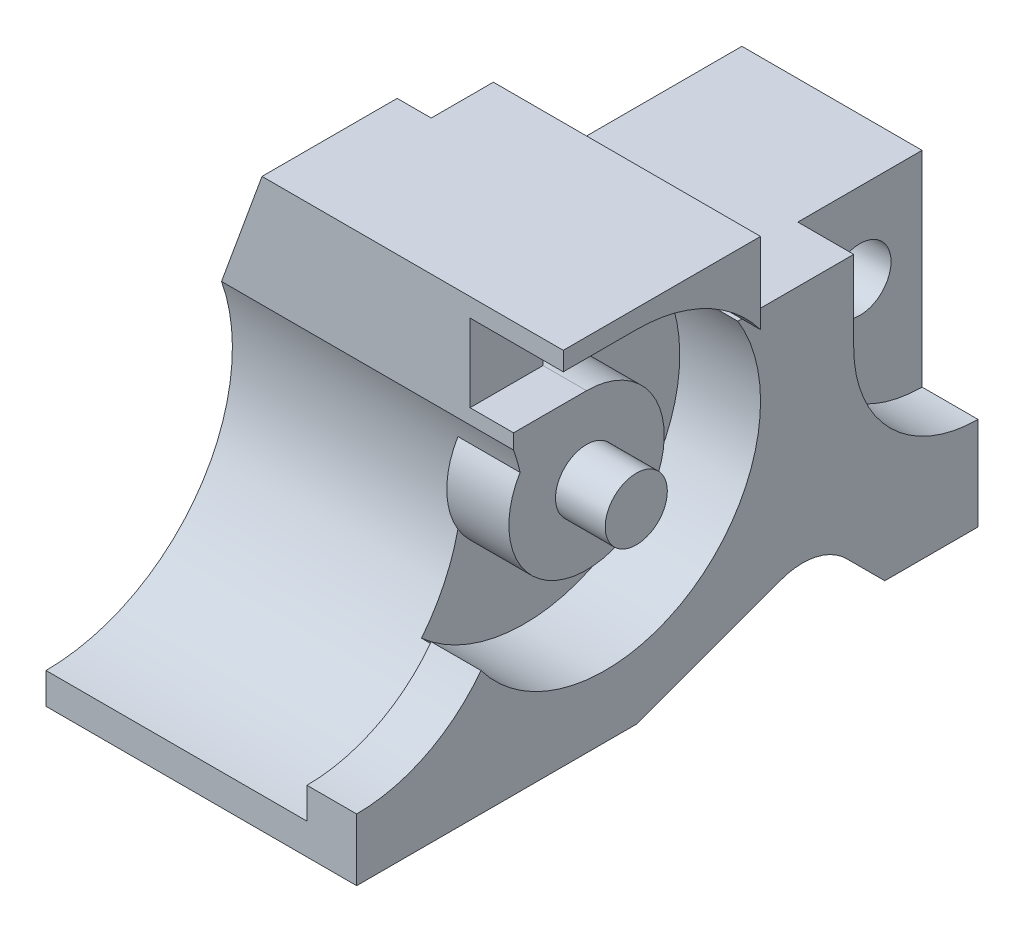
ISO-10303-21;
HEADER;
FILE_DESCRIPTION(('STEP AP214'),'2;1');
FILE_NAME('part.step','',(''),(''),'','','');
FILE_SCHEMA(('AUTOMOTIVE_DESIGN { 1 0 10303 214 1 1 1 1 }'));
ENDSEC;
DATA;
#1=APPLICATION_CONTEXT('core data for automotive mechanical design processes');
#2=APPLICATION_PROTOCOL_DEFINITION('international standard','automotive_design',2000,#1);
#3=PRODUCT_CONTEXT('',#1,'mechanical');
#4=PRODUCT('Part','Part','',(#3));
#5=PRODUCT_RELATED_PRODUCT_CATEGORY('part','',(#4));
#6=PRODUCT_DEFINITION_FORMATION('','',#4);
#7=PRODUCT_DEFINITION_CONTEXT('part definition',#1,'design');
#8=PRODUCT_DEFINITION('design','',#6,#7);
#9=PRODUCT_DEFINITION_SHAPE('','',#8);
#10=(LENGTH_UNIT() NAMED_UNIT(*) SI_UNIT(.MILLI.,.METRE.));
#11=(NAMED_UNIT(*) PLANE_ANGLE_UNIT() SI_UNIT($,.RADIAN.));
#12=(NAMED_UNIT(*) SI_UNIT($,.STERADIAN.) SOLID_ANGLE_UNIT());
#13=UNCERTAINTY_MEASURE_WITH_UNIT(LENGTH_MEASURE(1.E-05),#10,'distance_accuracy_value','');
#14=(GEOMETRIC_REPRESENTATION_CONTEXT(3) GLOBAL_UNCERTAINTY_ASSIGNED_CONTEXT((#13)) GLOBAL_UNIT_ASSIGNED_CONTEXT((#10,
#11,#12)) REPRESENTATION_CONTEXT('',''));
#15=CARTESIAN_POINT('',(0.,0.,0.));
#16=DIRECTION('',(0.,0.,1.));
#17=DIRECTION('',(1.,0.,0.));
#18=AXIS2_PLACEMENT_3D('',#15,#16,#17);
#19=CARTESIAN_POINT('',(12.,35.,-40.));
#20=DIRECTION('',(0.,0.,1.));
#21=DIRECTION('',(1.,0.,0.));
#22=AXIS2_PLACEMENT_3D('',#19,#20,#21);
#23=PLANE('',#22);
#24=DIRECTION('',(0.,-1.,0.));
#25=VECTOR('',#24,1.);
#26=CARTESIAN_POINT('',(15.,47.5,-40.));
#27=LINE('',#26,#25);
#28=CARTESIAN_POINT('',(15.,60.,-40.));
#29=VERTEX_POINT('',#28);
#30=CARTESIAN_POINT('',(15.,47.5,-40.));
#31=VERTEX_POINT('',#30);
#32=EDGE_CURVE('E259',#29,#31,#27,.T.);
#33=ORIENTED_EDGE('',*,*,#32,.T.);
#34=DIRECTION('',(-1.,0.,0.));
#35=VECTOR('',#34,1.);
#36=CARTESIAN_POINT('',(22.,47.5,-40.));
#37=LINE('',#36,#35);
#38=CARTESIAN_POINT('',(12.,47.5,-40.));
#39=VERTEX_POINT('',#38);
#40=EDGE_CURVE('E53',#39,#31,#37,.F.);
#41=ORIENTED_EDGE('',*,*,#40,.F.);
#42=DIRECTION('',(0.,-1.,0.));
#43=VECTOR('',#42,1.);
#44=CARTESIAN_POINT('',(12.,35.,-40.));
#45=LINE('',#44,#43);
#46=CARTESIAN_POINT('',(12.,60.,-40.));
#47=VERTEX_POINT('',#46);
#48=EDGE_CURVE('E308',#47,#39,#45,.T.);
#49=ORIENTED_EDGE('',*,*,#48,.F.);
#50=DIRECTION('',(1.,0.,0.));
#51=VECTOR('',#50,1.);
#52=CARTESIAN_POINT('',(12.,60.,-40.));
#53=LINE('',#52,#51);
#54=EDGE_CURVE('E312',#47,#29,#53,.T.);
#55=ORIENTED_EDGE('',*,*,#54,.T.);
#56=EDGE_LOOP('',(#33,#41,#49,#55));
#57=FACE_BOUND('',#56,.T.);
#58=ADVANCED_FACE('F46',(#57),#23,.F.);
#59=CARTESIAN_POINT('',(-25.,35.,0.));
#60=DIRECTION('',(1.,0.,0.));
#61=DIRECTION('',(0.,0.,-1.));
#62=AXIS2_PLACEMENT_3D('',#59,#60,#61);
#63=CYLINDRICAL_SURFACE('',#62,30.);
#64=CARTESIAN_POINT('',(22.,35.,0.));
#65=DIRECTION('',(-1.,0.,0.));
#66=DIRECTION('',(0.,0.,-1.));
#67=AXIS2_PLACEMENT_3D('',#64,#65,#66);
#68=CIRCLE('',#67,30.);
#69=CARTESIAN_POINT('',(22.,45.0964102531544,-28.25));
#70=VERTEX_POINT('',#69);
#71=CARTESIAN_POINT('',(22.,41.4570206159168,-29.296875));
#72=VERTEX_POINT('',#71);
#73=EDGE_CURVE('E274',#70,#72,#68,.T.);
#74=ORIENTED_EDGE('',*,*,#73,.F.);
#75=DIRECTION('',(1.,0.,0.));
#76=VECTOR('',#75,1.);
#77=CARTESIAN_POINT('',(-25.,45.0964102531544,-28.25));
#78=LINE('',#77,#76);
#79=CARTESIAN_POINT('',(-25.,45.0964102531544,-28.25));
#80=VERTEX_POINT('',#79);
#81=EDGE_CURVE('E68',#70,#80,#78,.F.);
#82=ORIENTED_EDGE('',*,*,#81,.T.);
#83=CARTESIAN_POINT('',(-25.,35.,0.));
#84=DIRECTION('',(1.,0.,0.));
#85=DIRECTION('',(0.,0.,-1.));
#86=AXIS2_PLACEMENT_3D('',#83,#84,#85);
#87=CIRCLE('',#86,30.);
#88=CARTESIAN_POINT('',(-25.,5.,0.));
#89=VERTEX_POINT('',#88);
#90=EDGE_CURVE('E348',#89,#80,#87,.T.);
#91=ORIENTED_EDGE('',*,*,#90,.F.);
#92=DIRECTION('',(1.,0.,0.));
#93=VECTOR('',#92,1.);
#94=CARTESIAN_POINT('',(-25.,5.,0.));
#95=LINE('',#94,#93);
#96=CARTESIAN_POINT('',(17.,5.,0.));
#97=VERTEX_POINT('',#96);
#98=EDGE_CURVE('E355',#89,#97,#95,.T.);
#99=ORIENTED_EDGE('',*,*,#98,.T.);
#100=CARTESIAN_POINT('',(17.,35.,0.));
#101=DIRECTION('',(1.,0.,0.));
#102=DIRECTION('',(0.,0.,-1.));
#103=AXIS2_PLACEMENT_3D('',#100,#101,#102);
#104=CIRCLE('',#103,30.);
#105=CARTESIAN_POINT('',(17.,16.2734521667767,-23.4375));
#106=VERTEX_POINT('',#105);
#107=EDGE_CURVE('E351',#97,#106,#104,.T.);
#108=ORIENTED_EDGE('',*,*,#107,.T.);
#109=DIRECTION('',(1.,0.,0.));
#110=VECTOR('',#109,1.);
#111=CARTESIAN_POINT('',(18.5,16.2734521667767,-23.4375));
#112=LINE('',#111,#110);
#113=CARTESIAN_POINT('',(12.,16.2734521667767,-23.4375));
#114=VERTEX_POINT('',#113);
#115=EDGE_CURVE('E314',#106,#114,#112,.F.);
#116=ORIENTED_EDGE('',*,*,#115,.T.);
#117=CARTESIAN_POINT('',(12.,35.,0.));
#118=DIRECTION('',(1.,0.,0.));
#119=DIRECTION('',(0.,0.,-1.));
#120=AXIS2_PLACEMENT_3D('',#117,#118,#119);
#121=CIRCLE('',#120,30.);
#122=CARTESIAN_POINT('',(12.,28.5429793840832,-29.296875));
#123=VERTEX_POINT('',#122);
#124=EDGE_CURVE('E476',#123,#114,#121,.F.);
#125=ORIENTED_EDGE('',*,*,#124,.F.);
#126=CARTESIAN_POINT('',(12.,41.4570206159168,-29.296875));
#127=VERTEX_POINT('',#126);
#128=EDGE_CURVE('E480',#127,#123,#121,.F.);
#129=ORIENTED_EDGE('',*,*,#128,.F.);
#130=DIRECTION('',(-1.,0.,0.));
#131=VECTOR('',#130,1.);
#132=CARTESIAN_POINT('',(17.,41.4570206159168,-29.296875));
#133=LINE('',#132,#131);
#134=EDGE_CURVE('E299',#72,#127,#133,.T.);
#135=ORIENTED_EDGE('',*,*,#134,.F.);
#136=EDGE_LOOP('',(#74,#82,#91,#99,#108,#116,#125,#129,#135));
#137=FACE_BOUND('',#136,.T.);
#138=ADVANCED_FACE('F521',(#137),#63,.F.);
#139=CARTESIAN_POINT('',(25.,63.,0.));
#140=DIRECTION('',(0.,1.,0.));
#141=DIRECTION('',(0.,0.,1.));
#142=AXIS2_PLACEMENT_3D('',#139,#140,#141);
#143=PLANE('',#142);
#144=DIRECTION('',(1.,0.,0.));
#145=VECTOR('',#144,1.);
#146=CARTESIAN_POINT('',(-25.,63.,-50.));
#147=LINE('',#146,#145);
#148=CARTESIAN_POINT('',(-18.4836262456348,63.,-50.));
#149=VERTEX_POINT('',#148);
#150=CARTESIAN_POINT('',(-13.,63.,-50.));
#151=VERTEX_POINT('',#150);
#152=EDGE_CURVE('E385',#149,#151,#147,.T.);
#153=ORIENTED_EDGE('',*,*,#152,.F.);
#154=DIRECTION('',(0.,0.,1.));
#155=VECTOR('',#154,1.);
#156=CARTESIAN_POINT('',(-18.4836262456348,63.,-100.));
#157=LINE('',#156,#155);
#158=CARTESIAN_POINT('',(-18.4836262456348,63.,-28.25));
#159=VERTEX_POINT('',#158);
#160=EDGE_CURVE('E332',#149,#159,#157,.T.);
#161=ORIENTED_EDGE('',*,*,#160,.T.);
#162=DIRECTION('',(-1.,0.,0.));
#163=VECTOR('',#162,1.);
#164=CARTESIAN_POINT('',(25.,63.,-28.25));
#165=LINE('',#164,#163);
#166=CARTESIAN_POINT('',(30.,63.,-28.25));
#167=VERTEX_POINT('',#166);
#168=EDGE_CURVE('E338',#167,#159,#165,.T.);
#169=ORIENTED_EDGE('',*,*,#168,.F.);
#170=DIRECTION('',(0.,0.,1.));
#171=VECTOR('',#170,1.);
#172=CARTESIAN_POINT('',(30.,63.,-28.25));
#173=LINE('',#172,#171);
#174=CARTESIAN_POINT('',(30.,63.,-60.));
#175=VERTEX_POINT('',#174);
#176=EDGE_CURVE('E273',#175,#167,#173,.T.);
#177=ORIENTED_EDGE('',*,*,#176,.F.);
#178=DIRECTION('',(1.,0.,0.));
#179=VECTOR('',#178,1.);
#180=CARTESIAN_POINT('',(-13.,63.,-60.));
#181=LINE('',#180,#179);
#182=CARTESIAN_POINT('',(-13.,63.,-60.));
#183=VERTEX_POINT('',#182);
#184=EDGE_CURVE('E370',#183,#175,#181,.T.);
#185=ORIENTED_EDGE('',*,*,#184,.F.);
#186=DIRECTION('',(0.,0.,-1.));
#187=VECTOR('',#186,1.);
#188=CARTESIAN_POINT('',(-13.,63.,-100.));
#189=LINE('',#188,#187);
#190=EDGE_CURVE('E389',#151,#183,#189,.T.);
#191=ORIENTED_EDGE('',*,*,#190,.F.);
#192=EDGE_LOOP('',(#153,#161,#169,#177,#185,#191));
#193=FACE_BOUND('',#192,.T.);
#194=ADVANCED_FACE('F503',(#193),#143,.T.);
#195=CARTESIAN_POINT('',(-25.,0.,0.));
#196=DIRECTION('',(1.,0.,0.));
#197=DIRECTION('',(0.,0.,-1.));
#198=AXIS2_PLACEMENT_3D('',#195,#196,#197);
#199=PLANE('',#198);
#200=DIRECTION('',(0.,0.,1.));
#201=VECTOR('',#200,1.);
#202=CARTESIAN_POINT('',(-25.,45.0964102531544,-100.));
#203=LINE('',#202,#201);
#204=CARTESIAN_POINT('',(-25.,45.0964102531544,-50.));
#205=VERTEX_POINT('',#204);
#206=EDGE_CURVE('E331',#205,#80,#203,.T.);
#207=ORIENTED_EDGE('',*,*,#206,.F.);
#208=DIRECTION('',(0.,-1.,0.));
#209=VECTOR('',#208,1.);
#210=CARTESIAN_POINT('',(-25.,0.,-50.));
#211=LINE('',#210,#209);
#212=CARTESIAN_POINT('',(-25.,1.81985117133101,-50.));
#213=VERTEX_POINT('',#212);
#214=EDGE_CURVE('E462',#205,#213,#211,.T.);
#215=ORIENTED_EDGE('',*,*,#214,.T.);
#216=DIRECTION('',(0.,0.34202014332567,-0.939692620785908));
#217=VECTOR('',#216,1.);
#218=CARTESIAN_POINT('',(-25.,-14.4627212179472,-5.26400002982302));
#219=LINE('',#218,#217);
#220=CARTESIAN_POINT('',(-25.,0.,-45.));
#221=VERTEX_POINT('',#220);
#222=EDGE_CURVE('E428',#221,#213,#219,.T.);
#223=ORIENTED_EDGE('',*,*,#222,.F.);
#224=DIRECTION('',(0.,0.,-1.));
#225=VECTOR('',#224,1.);
#226=CARTESIAN_POINT('',(-25.,0.,0.));
#227=LINE('',#226,#225);
#228=CARTESIAN_POINT('',(-25.,0.,0.));
#229=VERTEX_POINT('',#228);
#230=EDGE_CURVE('E444',#229,#221,#227,.T.);
#231=ORIENTED_EDGE('',*,*,#230,.F.);
#232=DIRECTION('',(0.,1.,0.));
#233=VECTOR('',#232,1.);
#234=CARTESIAN_POINT('',(-25.,0.,0.));
#235=LINE('',#234,#233);
#236=EDGE_CURVE('E419',#229,#89,#235,.T.);
#237=ORIENTED_EDGE('',*,*,#236,.T.);
#238=ORIENTED_EDGE('',*,*,#90,.T.);
#239=EDGE_LOOP('',(#207,#215,#223,#231,#237,#238));
#240=FACE_BOUND('',#239,.T.);
#241=ADVANCED_FACE('F519',(#240),#199,.F.);
#242=CARTESIAN_POINT('',(-25.,0.,-50.));
#243=DIRECTION('',(0.,0.,1.));
#244=DIRECTION('',(1.,0.,0.));
#245=AXIS2_PLACEMENT_3D('',#242,#243,#244);
#246=PLANE('',#245);
#247=DIRECTION('',(-0.342020143325663,-0.939692620785911,0.));
#248=VECTOR('',#247,1.);
#249=CARTESIAN_POINT('',(-39.4937068760341,5.2752778870557,-50.));
#250=LINE('',#249,#248);
#251=EDGE_CURVE('E336',#149,#205,#250,.T.);
#252=ORIENTED_EDGE('',*,*,#251,.F.);
#253=ORIENTED_EDGE('',*,*,#152,.T.);
#254=DIRECTION('',(0.,1.,0.));
#255=VECTOR('',#254,1.);
#256=CARTESIAN_POINT('',(-13.,0.,-50.));
#257=LINE('',#256,#255);
#258=CARTESIAN_POINT('',(-13.,1.81985117133101,-50.));
#259=VERTEX_POINT('',#258);
#260=EDGE_CURVE('E388',#259,#151,#257,.T.);
#261=ORIENTED_EDGE('',*,*,#260,.F.);
#262=DIRECTION('',(1.,0.,0.));
#263=VECTOR('',#262,1.);
#264=CARTESIAN_POINT('',(25.,1.81985117133101,-50.));
#265=LINE('',#264,#263);
#266=EDGE_CURVE('E393',#213,#259,#265,.T.);
#267=ORIENTED_EDGE('',*,*,#266,.F.);
#268=ORIENTED_EDGE('',*,*,#214,.F.);
#269=EDGE_LOOP('',(#252,#253,#261,#267,#268));
#270=FACE_BOUND('',#269,.T.);
#271=ADVANCED_FACE('F515',(#270),#246,.F.);
#272=CARTESIAN_POINT('',(25.,63.,-28.25));
#273=DIRECTION('',(0.,0.,-1.));
#274=DIRECTION('',(0.,1.,0.));
#275=AXIS2_PLACEMENT_3D('',#272,#273,#274);
#276=PLANE('',#275);
#277=DIRECTION('',(0.,-1.,0.));
#278=VECTOR('',#277,1.);
#279=CARTESIAN_POINT('',(22.,47.5,-28.25));
#280=LINE('',#279,#278);
#281=CARTESIAN_POINT('',(22.,47.5,-28.25));
#282=VERTEX_POINT('',#281);
#283=EDGE_CURVE('E287',#282,#70,#280,.T.);
#284=ORIENTED_EDGE('',*,*,#283,.F.);
#285=DIRECTION('',(1.,0.,0.));
#286=VECTOR('',#285,1.);
#287=CARTESIAN_POINT('',(-5.15553846429776,47.5,-28.25));
#288=LINE('',#287,#286);
#289=CARTESIAN_POINT('',(15.,47.5,-28.25));
#290=VERTEX_POINT('',#289);
#291=EDGE_CURVE('E265',#290,#282,#288,.T.);
#292=ORIENTED_EDGE('',*,*,#291,.F.);
#293=DIRECTION('',(0.,1.,0.));
#294=VECTOR('',#293,1.);
#295=CARTESIAN_POINT('',(15.,60.,-28.25));
#296=LINE('',#295,#294);
#297=CARTESIAN_POINT('',(15.,60.,-28.25));
#298=VERTEX_POINT('',#297);
#299=EDGE_CURVE('E251',#290,#298,#296,.T.);
#300=ORIENTED_EDGE('',*,*,#299,.T.);
#301=DIRECTION('',(-1.,0.,0.));
#302=VECTOR('',#301,1.);
#303=CARTESIAN_POINT('',(64.3083444660333,60.,-28.25));
#304=LINE('',#303,#302);
#305=CARTESIAN_POINT('',(30.,60.,-28.25));
#306=VERTEX_POINT('',#305);
#307=EDGE_CURVE('E238',#306,#298,#304,.T.);
#308=ORIENTED_EDGE('',*,*,#307,.F.);
#309=DIRECTION('',(0.,-1.,0.));
#310=VECTOR('',#309,1.);
#311=CARTESIAN_POINT('',(30.,60.,-28.25));
#312=LINE('',#311,#310);
#313=EDGE_CURVE('E275',#167,#306,#312,.T.);
#314=ORIENTED_EDGE('',*,*,#313,.F.);
#315=ORIENTED_EDGE('',*,*,#168,.T.);
#316=DIRECTION('',(-0.342020143325663,-0.939692620785911,0.));
#317=VECTOR('',#316,1.);
#318=CARTESIAN_POINT('',(-18.4836262456348,63.,-28.25));
#319=LINE('',#318,#317);
#320=EDGE_CURVE('E329',#159,#80,#319,.T.);
#321=ORIENTED_EDGE('',*,*,#320,.T.);
#322=ORIENTED_EDGE('',*,*,#81,.F.);
#323=EDGE_LOOP('',(#284,#292,#300,#308,#314,#315,#321,#322));
#324=FACE_BOUND('',#323,.T.);
#325=ADVANCED_FACE('F261',(#324),#276,.F.);
#326=CARTESIAN_POINT('',(25.,0.,0.));
#327=DIRECTION('',(1.,0.,0.));
#328=DIRECTION('',(0.,0.,-1.));
#329=AXIS2_PLACEMENT_3D('',#326,#327,#328);
#330=PLANE('',#329);
#331=CARTESIAN_POINT('',(25.,35.,-40.));
#332=DIRECTION('',(1.,0.,0.));
#333=DIRECTION('',(0.,0.,-1.));
#334=AXIS2_PLACEMENT_3D('',#331,#332,#333);
#335=CIRCLE('',#334,25.);
#336=CARTESIAN_POINT('',(25.,20.,-20.));
#337=VERTEX_POINT('',#336);
#338=CARTESIAN_POINT('',(25.,48.,-61.3541565040626));
#339=VERTEX_POINT('',#338);
#340=EDGE_CURVE('E302',#337,#339,#335,.T.);
#341=ORIENTED_EDGE('',*,*,#340,.F.);
#342=CARTESIAN_POINT('',(25.,35.,0.));
#343=DIRECTION('',(1.,0.,0.));
#344=DIRECTION('',(0.,0.,-1.));
#345=AXIS2_PLACEMENT_3D('',#342,#343,#344);
#346=CIRCLE('',#345,25.);
#347=CARTESIAN_POINT('',(25.,10.,0.));
#348=VERTEX_POINT('',#347);
#349=EDGE_CURVE('E342',#348,#337,#346,.T.);
#350=ORIENTED_EDGE('',*,*,#349,.F.);
#351=DIRECTION('',(0.,1.,0.));
#352=VECTOR('',#351,1.);
#353=CARTESIAN_POINT('',(25.,0.,0.));
#354=LINE('',#353,#352);
#355=CARTESIAN_POINT('',(25.,0.,0.));
#356=VERTEX_POINT('',#355);
#357=EDGE_CURVE('E434',#356,#348,#354,.T.);
#358=ORIENTED_EDGE('',*,*,#357,.F.);
#359=DIRECTION('',(0.,0.,-1.));
#360=VECTOR('',#359,1.);
#361=CARTESIAN_POINT('',(25.,0.,0.));
#362=LINE('',#361,#360);
#363=CARTESIAN_POINT('',(25.,0.,-45.));
#364=VERTEX_POINT('',#363);
#365=EDGE_CURVE('E438',#356,#364,#362,.T.);
#366=ORIENTED_EDGE('',*,*,#365,.T.);
#367=DIRECTION('',(0.,0.34202014332567,-0.939692620785908));
#368=VECTOR('',#367,1.);
#369=CARTESIAN_POINT('',(25.,-14.4627212179472,-5.26400002982302));
#370=LINE('',#369,#368);
#371=CARTESIAN_POINT('',(25.,8.49493821780103,-68.3396509330703));
#372=VERTEX_POINT('',#371);
#373=EDGE_CURVE('E439',#364,#372,#370,.T.);
#374=ORIENTED_EDGE('',*,*,#373,.T.);
#375=CARTESIAN_POINT('',(25.,-0.901987990058065,-71.7598523663271));
#376=DIRECTION('',(1.,0.,0.));
#377=DIRECTION('',(0.,0.,-1.));
#378=AXIS2_PLACEMENT_3D('',#375,#376,#377);
#379=CIRCLE('',#378,10.);
#380=CARTESIAN_POINT('',(25.,6.16907982180745,-78.8309201781925));
#381=VERTEX_POINT('',#380);
#382=EDGE_CURVE('E422',#381,#372,#379,.T.);
#383=ORIENTED_EDGE('',*,*,#382,.F.);
#384=DIRECTION('',(0.,0.707106781186544,0.707106781186551));
#385=VECTOR('',#384,1.);
#386=CARTESIAN_POINT('',(25.,42.5,-42.4999999999995));
#387=LINE('',#386,#385);
#388=CARTESIAN_POINT('',(25.,0.,-85.));
#389=VERTEX_POINT('',#388);
#390=EDGE_CURVE('E424',#389,#381,#387,.T.);
#391=ORIENTED_EDGE('',*,*,#390,.F.);
#392=DIRECTION('',(0.,0.,1.));
#393=VECTOR('',#392,1.);
#394=CARTESIAN_POINT('',(25.,0.,0.));
#395=LINE('',#394,#393);
#396=CARTESIAN_POINT('',(25.,0.,-100.));
#397=VERTEX_POINT('',#396);
#398=EDGE_CURVE('E429',#397,#389,#395,.T.);
#399=ORIENTED_EDGE('',*,*,#398,.F.);
#400=DIRECTION('',(0.,1.,0.));
#401=VECTOR('',#400,1.);
#402=CARTESIAN_POINT('',(25.,0.,-100.));
#403=LINE('',#402,#401);
#404=CARTESIAN_POINT('',(25.,15.,-100.));
#405=VERTEX_POINT('',#404);
#406=EDGE_CURVE('E435',#397,#405,#403,.T.);
#407=ORIENTED_EDGE('',*,*,#406,.T.);
#408=CARTESIAN_POINT('',(25.,35.,-100.));
#409=DIRECTION('',(1.,0.,0.));
#410=DIRECTION('',(0.,0.,-1.));
#411=AXIS2_PLACEMENT_3D('',#408,#409,#410);
#412=CIRCLE('',#411,20.);
#413=CARTESIAN_POINT('',(25.,35.,-80.));
#414=VERTEX_POINT('',#413);
#415=EDGE_CURVE('E409',#414,#405,#412,.T.);
#416=ORIENTED_EDGE('',*,*,#415,.F.);
#417=DIRECTION('',(0.,-1.,0.));
#418=VECTOR('',#417,1.);
#419=CARTESIAN_POINT('',(25.,35.,-80.));
#420=LINE('',#419,#418);
#421=CARTESIAN_POINT('',(25.,48.,-80.));
#422=VERTEX_POINT('',#421);
#423=EDGE_CURVE('E401',#422,#414,#420,.T.);
#424=ORIENTED_EDGE('',*,*,#423,.F.);
#425=DIRECTION('',(0.,0.,-1.));
#426=VECTOR('',#425,1.);
#427=CARTESIAN_POINT('',(25.,48.,-100.));
#428=LINE('',#427,#426);
#429=EDGE_CURVE('E369',#339,#422,#428,.T.);
#430=ORIENTED_EDGE('',*,*,#429,.F.);
#431=EDGE_LOOP('',(#341,#350,#358,#366,#374,#383,#391,#399,#407,#416,#424,#430));
#432=FACE_BOUND('',#431,.T.);
#433=ADVANCED_FACE('F555',(#432),#330,.T.);
#434=CARTESIAN_POINT('',(17.,0.,0.));
#435=DIRECTION('',(1.,0.,0.));
#436=DIRECTION('',(0.,0.,-1.));
#437=AXIS2_PLACEMENT_3D('',#434,#435,#436);
#438=PLANE('',#437);
#439=CARTESIAN_POINT('',(17.,35.,0.));
#440=DIRECTION('',(1.,0.,0.));
#441=DIRECTION('',(0.,0.,-1.));
#442=AXIS2_PLACEMENT_3D('',#439,#440,#441);
#443=CIRCLE('',#442,25.);
#444=CARTESIAN_POINT('',(17.,10.,0.));
#445=VERTEX_POINT('',#444);
#446=CARTESIAN_POINT('',(17.,20.,-20.));
#447=VERTEX_POINT('',#446);
#448=EDGE_CURVE('E468',#445,#447,#443,.T.);
#449=ORIENTED_EDGE('',*,*,#448,.T.);
#450=CARTESIAN_POINT('',(17.,35.,-40.));
#451=DIRECTION('',(1.,0.,0.));
#452=DIRECTION('',(0.,0.,-1.));
#453=AXIS2_PLACEMENT_3D('',#450,#451,#452);
#454=CIRCLE('',#453,25.);
#455=EDGE_CURVE('E63',#447,#106,#454,.T.);
#456=ORIENTED_EDGE('',*,*,#455,.T.);
#457=ORIENTED_EDGE('',*,*,#107,.F.);
#458=DIRECTION('',(0.,-1.,0.));
#459=VECTOR('',#458,1.);
#460=CARTESIAN_POINT('',(17.,0.,0.));
#461=LINE('',#460,#459);
#462=EDGE_CURVE('E347',#445,#97,#461,.T.);
#463=ORIENTED_EDGE('',*,*,#462,.F.);
#464=EDGE_LOOP('',(#449,#456,#457,#463));
#465=FACE_BOUND('',#464,.T.);
#466=ADVANCED_FACE('F526',(#465),#438,.F.);
#467=CARTESIAN_POINT('',(25.,0.,0.));
#468=DIRECTION('',(0.,0.,1.));
#469=DIRECTION('',(1.,0.,0.));
#470=AXIS2_PLACEMENT_3D('',#467,#468,#469);
#471=PLANE('',#470);
#472=DIRECTION('',(1.,0.,0.));
#473=VECTOR('',#472,1.);
#474=CARTESIAN_POINT('',(-25.,10.,0.));
#475=LINE('',#474,#473);
#476=EDGE_CURVE('E346',#445,#348,#475,.T.);
#477=ORIENTED_EDGE('',*,*,#476,.F.);
#478=ORIENTED_EDGE('',*,*,#462,.T.);
#479=ORIENTED_EDGE('',*,*,#98,.F.);
#480=ORIENTED_EDGE('',*,*,#236,.F.);
#481=DIRECTION('',(-1.,0.,0.));
#482=VECTOR('',#481,1.);
#483=CARTESIAN_POINT('',(25.,0.,0.));
#484=LINE('',#483,#482);
#485=EDGE_CURVE('E455',#356,#229,#484,.T.);
#486=ORIENTED_EDGE('',*,*,#485,.F.);
#487=ORIENTED_EDGE('',*,*,#357,.T.);
#488=EDGE_LOOP('',(#477,#478,#479,#480,#486,#487));
#489=FACE_BOUND('',#488,.T.);
#490=ADVANCED_FACE('F524',(#489),#471,.T.);
#491=CARTESIAN_POINT('',(25.,0.,-100.));
#492=DIRECTION('',(0.,0.,1.));
#493=DIRECTION('',(1.,0.,0.));
#494=AXIS2_PLACEMENT_3D('',#491,#492,#493);
#495=PLANE('',#494);
#496=DIRECTION('',(-1.,0.,0.));
#497=VECTOR('',#496,1.);
#498=CARTESIAN_POINT('',(-13.,48.,-100.));
#499=LINE('',#498,#497);
#500=CARTESIAN_POINT('',(16.,48.,-100.));
#501=VERTEX_POINT('',#500);
#502=CARTESIAN_POINT('',(-13.,48.,-100.));
#503=VERTEX_POINT('',#502);
#504=EDGE_CURVE('E375',#501,#503,#499,.T.);
#505=ORIENTED_EDGE('',*,*,#504,.F.);
#506=DIRECTION('',(0.,1.,0.));
#507=VECTOR('',#506,1.);
#508=CARTESIAN_POINT('',(16.,15.,-100.));
#509=LINE('',#508,#507);
#510=CARTESIAN_POINT('',(16.,15.,-100.));
#511=VERTEX_POINT('',#510);
#512=EDGE_CURVE('E406',#511,#501,#509,.T.);
#513=ORIENTED_EDGE('',*,*,#512,.F.);
#514=DIRECTION('',(1.,0.,0.));
#515=VECTOR('',#514,1.);
#516=CARTESIAN_POINT('',(16.,15.,-100.));
#517=LINE('',#516,#515);
#518=EDGE_CURVE('E418',#511,#405,#517,.T.);
#519=ORIENTED_EDGE('',*,*,#518,.T.);
#520=ORIENTED_EDGE('',*,*,#406,.F.);
#521=DIRECTION('',(-1.,0.,0.));
#522=VECTOR('',#521,1.);
#523=CARTESIAN_POINT('',(25.,0.,-100.));
#524=LINE('',#523,#522);
#525=CARTESIAN_POINT('',(-13.,0.,-100.));
#526=VERTEX_POINT('',#525);
#527=EDGE_CURVE('E456',#397,#526,#524,.T.);
#528=ORIENTED_EDGE('',*,*,#527,.T.);
#529=DIRECTION('',(0.,1.,0.));
#530=VECTOR('',#529,1.);
#531=CARTESIAN_POINT('',(-13.,0.,-100.));
#532=LINE('',#531,#530);
#533=EDGE_CURVE('E391',#526,#503,#532,.T.);
#534=ORIENTED_EDGE('',*,*,#533,.T.);
#535=EDGE_LOOP('',(#505,#513,#519,#520,#528,#534));
#536=FACE_BOUND('',#535,.T.);
#537=ADVANCED_FACE('F606',(#536),#495,.F.);
#538=CARTESIAN_POINT('',(16.,35.,-80.));
#539=DIRECTION('',(0.,0.,1.));
#540=DIRECTION('',(0.,-1.,0.));
#541=AXIS2_PLACEMENT_3D('',#538,#539,#540);
#542=PLANE('',#541);
#543=DIRECTION('',(-1.,0.,0.));
#544=VECTOR('',#543,1.);
#545=CARTESIAN_POINT('',(16.,48.,-80.));
#546=LINE('',#545,#544);
#547=CARTESIAN_POINT('',(16.,48.,-80.));
#548=VERTEX_POINT('',#547);
#549=EDGE_CURVE('E379',#422,#548,#546,.T.);
#550=ORIENTED_EDGE('',*,*,#549,.F.);
#551=ORIENTED_EDGE('',*,*,#423,.T.);
#552=DIRECTION('',(1.,0.,0.));
#553=VECTOR('',#552,1.);
#554=CARTESIAN_POINT('',(16.,35.,-80.));
#555=LINE('',#554,#553);
#556=CARTESIAN_POINT('',(16.,35.,-80.));
#557=VERTEX_POINT('',#556);
#558=EDGE_CURVE('E412',#557,#414,#555,.T.);
#559=ORIENTED_EDGE('',*,*,#558,.F.);
#560=DIRECTION('',(0.,-1.,0.));
#561=VECTOR('',#560,1.);
#562=CARTESIAN_POINT('',(16.,35.,-80.));
#563=LINE('',#562,#561);
#564=EDGE_CURVE('E404',#548,#557,#563,.T.);
#565=ORIENTED_EDGE('',*,*,#564,.F.);
#566=EDGE_LOOP('',(#550,#551,#559,#565));
#567=FACE_BOUND('',#566,.T.);
#568=ADVANCED_FACE('F599',(#567),#542,.F.);
#569=CARTESIAN_POINT('',(16.,35.,-100.));
#570=DIRECTION('',(1.,0.,0.));
#571=DIRECTION('',(0.,0.,-1.));
#572=AXIS2_PLACEMENT_3D('',#569,#570,#571);
#573=PLANE('',#572);
#574=CARTESIAN_POINT('',(16.,35.,-90.));
#575=DIRECTION('',(1.,0.,0.));
#576=DIRECTION('',(0.,0.,-1.));
#577=AXIS2_PLACEMENT_3D('',#574,#575,#576);
#578=CIRCLE('',#577,5.00000000000001);
#579=CARTESIAN_POINT('',(16.,35.,-95.));
#580=VERTEX_POINT('',#579);
#581=EDGE_CURVE('E360',#580,#580,#578,.T.);
#582=ORIENTED_EDGE('',*,*,#581,.F.);
#583=EDGE_LOOP('',(#582));
#584=FACE_BOUND('',#583,.T.);
#585=ORIENTED_EDGE('',*,*,#512,.T.);
#586=DIRECTION('',(0.,0.,1.));
#587=VECTOR('',#586,1.);
#588=CARTESIAN_POINT('',(16.,48.,-100.));
#589=LINE('',#588,#587);
#590=EDGE_CURVE('E380',#501,#548,#589,.T.);
#591=ORIENTED_EDGE('',*,*,#590,.T.);
#592=ORIENTED_EDGE('',*,*,#564,.T.);
#593=CARTESIAN_POINT('',(16.,35.,-100.));
#594=DIRECTION('',(1.,0.,0.));
#595=DIRECTION('',(0.,0.,-1.));
#596=AXIS2_PLACEMENT_3D('',#593,#594,#595);
#597=CIRCLE('',#596,20.);
#598=EDGE_CURVE('E408',#557,#511,#597,.T.);
#599=ORIENTED_EDGE('',*,*,#598,.T.);
#600=EDGE_LOOP('',(#585,#591,#592,#599));
#601=FACE_BOUND('',#600,.T.);
#602=ADVANCED_FACE('F597',(#584,#601),#573,.T.);
#603=CARTESIAN_POINT('',(25.,-0.901987990058065,-71.7598523663271));
#604=DIRECTION('',(-1.,0.,0.));
#605=DIRECTION('',(0.,0.,1.));
#606=AXIS2_PLACEMENT_3D('',#603,#604,#605);
#607=CYLINDRICAL_SURFACE('',#606,10.);
#608=CARTESIAN_POINT('',(-13.,-0.901987990058065,-71.7598523663271));
#609=DIRECTION('',(1.,0.,0.));
#610=DIRECTION('',(0.,0.,-1.));
#611=AXIS2_PLACEMENT_3D('',#608,#609,#610);
#612=CIRCLE('',#611,10.);
#613=CARTESIAN_POINT('',(-13.,6.16907982180745,-78.8309201781925));
#614=VERTEX_POINT('',#613);
#615=CARTESIAN_POINT('',(-13.,8.49493821780102,-68.3396509330703));
#616=VERTEX_POINT('',#615);
#617=EDGE_CURVE('E399',#614,#616,#612,.T.);
#618=ORIENTED_EDGE('',*,*,#617,.F.);
#619=DIRECTION('',(-1.,0.,0.));
#620=VECTOR('',#619,1.);
#621=CARTESIAN_POINT('',(25.,6.16907982180745,-78.8309201781925));
#622=LINE('',#621,#620);
#623=EDGE_CURVE('E465',#381,#614,#622,.T.);
#624=ORIENTED_EDGE('',*,*,#623,.F.);
#625=ORIENTED_EDGE('',*,*,#382,.T.);
#626=DIRECTION('',(-1.,0.,0.));
#627=VECTOR('',#626,1.);
#628=CARTESIAN_POINT('',(25.,8.49493821780103,-68.3396509330703));
#629=LINE('',#628,#627);
#630=EDGE_CURVE('E445',#372,#616,#629,.T.);
#631=ORIENTED_EDGE('',*,*,#630,.T.);
#632=EDGE_LOOP('',(#618,#624,#625,#631));
#633=FACE_BOUND('',#632,.T.);
#634=ADVANCED_FACE('F48',(#633),#607,.F.);
#635=CARTESIAN_POINT('',(25.,42.5,-42.4999999999995));
#636=DIRECTION('',(0.,-0.707106781186551,0.707106781186544));
#637=DIRECTION('',(0.,-0.707106781186544,-0.707106781186551));
#638=AXIS2_PLACEMENT_3D('',#635,#636,#637);
#639=PLANE('',#638);
#640=DIRECTION('',(0.,0.707106781186544,0.707106781186551));
#641=VECTOR('',#640,1.);
#642=CARTESIAN_POINT('',(-13.,42.5,-42.4999999999995));
#643=LINE('',#642,#641);
#644=CARTESIAN_POINT('',(-13.,0.,-85.));
#645=VERTEX_POINT('',#644);
#646=EDGE_CURVE('E402',#645,#614,#643,.T.);
#647=ORIENTED_EDGE('',*,*,#646,.F.);
#648=DIRECTION('',(-1.,0.,0.));
#649=VECTOR('',#648,1.);
#650=CARTESIAN_POINT('',(25.,0.,-85.));
#651=LINE('',#650,#649);
#652=EDGE_CURVE('E458',#389,#645,#651,.T.);
#653=ORIENTED_EDGE('',*,*,#652,.F.);
#654=ORIENTED_EDGE('',*,*,#390,.T.);
#655=ORIENTED_EDGE('',*,*,#623,.T.);
#656=EDGE_LOOP('',(#647,#653,#654,#655));
#657=FACE_BOUND('',#656,.T.);
#658=ADVANCED_FACE('F625',(#657),#639,.T.);
#659=CARTESIAN_POINT('',(25.,0.,0.));
#660=DIRECTION('',(0.,-1.,0.));
#661=DIRECTION('',(0.,0.,-1.));
#662=AXIS2_PLACEMENT_3D('',#659,#660,#661);
#663=PLANE('',#662);
#664=DIRECTION('',(0.,0.,-1.));
#665=VECTOR('',#664,1.);
#666=CARTESIAN_POINT('',(-13.,0.,-100.));
#667=LINE('',#666,#665);
#668=EDGE_CURVE('E384',#645,#526,#667,.T.);
#669=ORIENTED_EDGE('',*,*,#668,.T.);
#670=ORIENTED_EDGE('',*,*,#527,.F.);
#671=ORIENTED_EDGE('',*,*,#398,.T.);
#672=ORIENTED_EDGE('',*,*,#652,.T.);
#673=EDGE_LOOP('',(#669,#670,#671,#672));
#674=FACE_BOUND('',#673,.T.);
#675=ADVANCED_FACE('F611',(#674),#663,.T.);
#676=CARTESIAN_POINT('',(25.,0.,0.));
#677=DIRECTION('',(0.,1.,0.));
#678=DIRECTION('',(0.,0.,1.));
#679=AXIS2_PLACEMENT_3D('',#676,#677,#678);
#680=PLANE('',#679);
#681=ORIENTED_EDGE('',*,*,#230,.T.);
#682=DIRECTION('',(-1.,0.,0.));
#683=VECTOR('',#682,1.);
#684=CARTESIAN_POINT('',(25.,0.,-45.));
#685=LINE('',#684,#683);
#686=EDGE_CURVE('E453',#364,#221,#685,.T.);
#687=ORIENTED_EDGE('',*,*,#686,.F.);
#688=ORIENTED_EDGE('',*,*,#365,.F.);
#689=ORIENTED_EDGE('',*,*,#485,.T.);
#690=EDGE_LOOP('',(#681,#687,#688,#689));
#691=FACE_BOUND('',#690,.T.);
#692=ADVANCED_FACE('F549',(#691),#680,.F.);
#693=CARTESIAN_POINT('',(25.,-14.4627212179472,-5.26400002982302));
#694=DIRECTION('',(0.,0.939692620785908,0.34202014332567));
#695=DIRECTION('',(0.,-0.34202014332567,0.939692620785908));
#696=AXIS2_PLACEMENT_3D('',#693,#694,#695);
#697=PLANE('',#696);
#698=ORIENTED_EDGE('',*,*,#266,.T.);
#699=DIRECTION('',(0.,0.34202014332567,-0.939692620785908));
#700=VECTOR('',#699,1.);
#701=CARTESIAN_POINT('',(-13.,-14.4627212179472,-5.26400002982302));
#702=LINE('',#701,#700);
#703=EDGE_CURVE('E470',#259,#616,#702,.T.);
#704=ORIENTED_EDGE('',*,*,#703,.T.);
#705=ORIENTED_EDGE('',*,*,#630,.F.);
#706=ORIENTED_EDGE('',*,*,#373,.F.);
#707=ORIENTED_EDGE('',*,*,#686,.T.);
#708=ORIENTED_EDGE('',*,*,#222,.T.);
#709=EDGE_LOOP('',(#698,#704,#705,#706,#707,#708));
#710=FACE_BOUND('',#709,.T.);
#711=ADVANCED_FACE('F542',(#710),#697,.F.);
#712=CARTESIAN_POINT('',(16.,35.,-100.));
#713=DIRECTION('',(1.,0.,0.));
#714=DIRECTION('',(0.,0.,-1.));
#715=AXIS2_PLACEMENT_3D('',#712,#713,#714);
#716=CYLINDRICAL_SURFACE('',#715,20.);
#717=ORIENTED_EDGE('',*,*,#415,.T.);
#718=ORIENTED_EDGE('',*,*,#518,.F.);
#719=ORIENTED_EDGE('',*,*,#598,.F.);
#720=ORIENTED_EDGE('',*,*,#558,.T.);
#721=EDGE_LOOP('',(#717,#718,#719,#720));
#722=FACE_BOUND('',#721,.T.);
#723=ADVANCED_FACE('F603',(#722),#716,.F.);
#724=CARTESIAN_POINT('',(-13.,0.,-100.));
#725=DIRECTION('',(1.,0.,0.));
#726=DIRECTION('',(0.,0.,-1.));
#727=AXIS2_PLACEMENT_3D('',#724,#725,#726);
#728=PLANE('',#727);
#729=CARTESIAN_POINT('',(-13.,35.,-90.));
#730=DIRECTION('',(1.,0.,0.));
#731=DIRECTION('',(0.,0.,-1.));
#732=AXIS2_PLACEMENT_3D('',#729,#730,#731);
#733=CIRCLE('',#732,5.00000000000001);
#734=CARTESIAN_POINT('',(-13.,35.,-95.));
#735=VERTEX_POINT('',#734);
#736=EDGE_CURVE('E365',#735,#735,#733,.T.);
#737=ORIENTED_EDGE('',*,*,#736,.T.);
#738=EDGE_LOOP('',(#737));
#739=FACE_BOUND('',#738,.T.);
#740=ORIENTED_EDGE('',*,*,#190,.T.);
#741=DIRECTION('',(0.,1.,0.));
#742=VECTOR('',#741,1.);
#743=CARTESIAN_POINT('',(-13.,48.,-60.));
#744=LINE('',#743,#742);
#745=CARTESIAN_POINT('',(-13.,48.,-60.));
#746=VERTEX_POINT('',#745);
#747=EDGE_CURVE('E372',#746,#183,#744,.T.);
#748=ORIENTED_EDGE('',*,*,#747,.F.);
#749=DIRECTION('',(0.,0.,1.));
#750=VECTOR('',#749,1.);
#751=CARTESIAN_POINT('',(-13.,48.,-100.));
#752=LINE('',#751,#750);
#753=EDGE_CURVE('E361',#503,#746,#752,.T.);
#754=ORIENTED_EDGE('',*,*,#753,.F.);
#755=ORIENTED_EDGE('',*,*,#533,.F.);
#756=ORIENTED_EDGE('',*,*,#668,.F.);
#757=ORIENTED_EDGE('',*,*,#646,.T.);
#758=ORIENTED_EDGE('',*,*,#617,.T.);
#759=ORIENTED_EDGE('',*,*,#703,.F.);
#760=ORIENTED_EDGE('',*,*,#260,.T.);
#761=EDGE_LOOP('',(#740,#748,#754,#755,#756,#757,#758,#759,#760));
#762=FACE_BOUND('',#761,.T.);
#763=ADVANCED_FACE('F541',(#739,#762),#728,.F.);
#764=CARTESIAN_POINT('',(0.,48.,0.));
#765=DIRECTION('',(0.,1.,0.));
#766=DIRECTION('',(0.,0.,1.));
#767=AXIS2_PLACEMENT_3D('',#764,#765,#766);
#768=PLANE('',#767);
#769=DIRECTION('',(1.,0.,0.));
#770=VECTOR('',#769,1.);
#771=CARTESIAN_POINT('',(12.,48.,-61.3541565040626));
#772=LINE('',#771,#770);
#773=CARTESIAN_POINT('',(12.,48.,-61.3541565040626));
#774=VERTEX_POINT('',#773);
#775=EDGE_CURVE('E322',#339,#774,#772,.F.);
#776=ORIENTED_EDGE('',*,*,#775,.F.);
#777=ORIENTED_EDGE('',*,*,#429,.T.);
#778=ORIENTED_EDGE('',*,*,#549,.T.);
#779=ORIENTED_EDGE('',*,*,#590,.F.);
#780=ORIENTED_EDGE('',*,*,#504,.T.);
#781=ORIENTED_EDGE('',*,*,#753,.T.);
#782=DIRECTION('',(1.,0.,0.));
#783=VECTOR('',#782,1.);
#784=CARTESIAN_POINT('',(-13.,48.,-60.));
#785=LINE('',#784,#783);
#786=CARTESIAN_POINT('',(12.,48.,-60.));
#787=VERTEX_POINT('',#786);
#788=EDGE_CURVE('E366',#746,#787,#785,.T.);
#789=ORIENTED_EDGE('',*,*,#788,.T.);
#790=DIRECTION('',(0.,0.,-1.));
#791=VECTOR('',#790,1.);
#792=CARTESIAN_POINT('',(12.,48.,0.));
#793=LINE('',#792,#791);
#794=EDGE_CURVE('E330',#787,#774,#793,.T.);
#795=ORIENTED_EDGE('',*,*,#794,.T.);
#796=EDGE_LOOP('',(#776,#777,#778,#779,#780,#781,#789,#795));
#797=FACE_BOUND('',#796,.T.);
#798=ADVANCED_FACE('F534',(#797),#768,.T.);
#799=CARTESIAN_POINT('',(-13.,48.,-60.));
#800=DIRECTION('',(0.,0.,1.));
#801=DIRECTION('',(1.,0.,0.));
#802=AXIS2_PLACEMENT_3D('',#799,#800,#801);
#803=PLANE('',#802);
#804=ORIENTED_EDGE('',*,*,#184,.T.);
#805=DIRECTION('',(0.,1.,0.));
#806=VECTOR('',#805,1.);
#807=CARTESIAN_POINT('',(30.,63.,-60.));
#808=LINE('',#807,#806);
#809=CARTESIAN_POINT('',(30.,50.,-60.));
#810=VERTEX_POINT('',#809);
#811=EDGE_CURVE('E277',#810,#175,#808,.T.);
#812=ORIENTED_EDGE('',*,*,#811,.F.);
#813=DIRECTION('',(1.,0.,0.));
#814=VECTOR('',#813,1.);
#815=CARTESIAN_POINT('',(12.,50.,-60.));
#816=LINE('',#815,#814);
#817=CARTESIAN_POINT('',(12.,50.,-60.));
#818=VERTEX_POINT('',#817);
#819=EDGE_CURVE('E318',#810,#818,#816,.F.);
#820=ORIENTED_EDGE('',*,*,#819,.T.);
#821=DIRECTION('',(0.,1.,0.));
#822=VECTOR('',#821,1.);
#823=CARTESIAN_POINT('',(12.,48.,-60.));
#824=LINE('',#823,#822);
#825=EDGE_CURVE('E321',#787,#818,#824,.T.);
#826=ORIENTED_EDGE('',*,*,#825,.F.);
#827=ORIENTED_EDGE('',*,*,#788,.F.);
#828=ORIENTED_EDGE('',*,*,#747,.T.);
#829=EDGE_LOOP('',(#804,#812,#820,#826,#827,#828));
#830=FACE_BOUND('',#829,.T.);
#831=ADVANCED_FACE('F540',(#830),#803,.F.);
#832=CARTESIAN_POINT('',(-25.,35.,-90.));
#833=DIRECTION('',(1.,0.,0.));
#834=DIRECTION('',(0.,0.,-1.));
#835=AXIS2_PLACEMENT_3D('',#832,#833,#834);
#836=CYLINDRICAL_SURFACE('',#835,5.00000000000001);
#837=ORIENTED_EDGE('',*,*,#581,.T.);
#838=EDGE_LOOP('',(#837));
#839=FACE_BOUND('',#838,.T.);
#840=ORIENTED_EDGE('',*,*,#736,.F.);
#841=EDGE_LOOP('',(#840));
#842=FACE_BOUND('',#841,.T.);
#843=ADVANCED_FACE('F556',(#839,#842),#836,.F.);
#844=CARTESIAN_POINT('',(-25.,35.,0.));
#845=DIRECTION('',(1.,0.,0.));
#846=DIRECTION('',(0.,0.,-1.));
#847=AXIS2_PLACEMENT_3D('',#844,#845,#846);
#848=CYLINDRICAL_SURFACE('',#847,25.);
#849=ORIENTED_EDGE('',*,*,#349,.T.);
#850=DIRECTION('',(1.,0.,0.));
#851=VECTOR('',#850,1.);
#852=CARTESIAN_POINT('',(12.,20.,-20.));
#853=LINE('',#852,#851);
#854=EDGE_CURVE('E311',#447,#337,#853,.T.);
#855=ORIENTED_EDGE('',*,*,#854,.F.);
#856=ORIENTED_EDGE('',*,*,#448,.F.);
#857=ORIENTED_EDGE('',*,*,#476,.T.);
#858=EDGE_LOOP('',(#849,#855,#856,#857));
#859=FACE_BOUND('',#858,.T.);
#860=ADVANCED_FACE('F558',(#859),#848,.F.);
#861=CARTESIAN_POINT('',(-18.4836262456348,63.,-100.));
#862=DIRECTION('',(-0.939692620785911,0.342020143325663,0.));
#863=DIRECTION('',(-0.342020143325663,-0.939692620785911,0.));
#864=AXIS2_PLACEMENT_3D('',#861,#862,#863);
#865=PLANE('',#864);
#866=ORIENTED_EDGE('',*,*,#251,.T.);
#867=ORIENTED_EDGE('',*,*,#206,.T.);
#868=ORIENTED_EDGE('',*,*,#320,.F.);
#869=ORIENTED_EDGE('',*,*,#160,.F.);
#870=EDGE_LOOP('',(#866,#867,#868,#869));
#871=FACE_BOUND('',#870,.T.);
#872=ADVANCED_FACE('F507',(#871),#865,.T.);
#873=CARTESIAN_POINT('',(12.,35.,-40.));
#874=DIRECTION('',(1.,0.,0.));
#875=DIRECTION('',(0.,0.,-1.));
#876=AXIS2_PLACEMENT_3D('',#873,#874,#875);
#877=PLANE('',#876);
#878=ORIENTED_EDGE('',*,*,#48,.T.);
#879=CARTESIAN_POINT('',(12.,35.,-40.));
#880=DIRECTION('',(1.,0.,0.));
#881=DIRECTION('',(0.,0.,-1.));
#882=AXIS2_PLACEMENT_3D('',#879,#880,#881);
#883=CIRCLE('',#882,12.5);
#884=EDGE_CURVE('E294',#123,#39,#883,.T.);
#885=ORIENTED_EDGE('',*,*,#884,.F.);
#886=ORIENTED_EDGE('',*,*,#124,.T.);
#887=CARTESIAN_POINT('',(12.,35.,-40.));
#888=DIRECTION('',(1.,0.,0.));
#889=DIRECTION('',(0.,0.,-1.));
#890=AXIS2_PLACEMENT_3D('',#887,#888,#889);
#891=CIRCLE('',#890,25.);
#892=EDGE_CURVE('E310',#114,#774,#891,.T.);
#893=ORIENTED_EDGE('',*,*,#892,.T.);
#894=ORIENTED_EDGE('',*,*,#794,.F.);
#895=ORIENTED_EDGE('',*,*,#825,.T.);
#896=EDGE_CURVE('E304',#818,#47,#891,.T.);
#897=ORIENTED_EDGE('',*,*,#896,.T.);
#898=EDGE_LOOP('',(#878,#885,#886,#893,#894,#895,#897));
#899=FACE_BOUND('',#898,.T.);
#900=ADVANCED_FACE('F490',(#899),#877,.T.);
#901=CARTESIAN_POINT('',(12.,35.,-40.));
#902=DIRECTION('',(1.,0.,0.));
#903=DIRECTION('',(0.,0.,-1.));
#904=AXIS2_PLACEMENT_3D('',#901,#902,#903);
#905=CYLINDRICAL_SURFACE('',#904,25.);
#906=ORIENTED_EDGE('',*,*,#819,.F.);
#907=CARTESIAN_POINT('',(30.,35.,-40.));
#908=DIRECTION('',(1.,0.,0.));
#909=DIRECTION('',(0.,0.,-1.));
#910=AXIS2_PLACEMENT_3D('',#907,#908,#909);
#911=CIRCLE('',#910,25.);
#912=CARTESIAN_POINT('',(30.,60.,-40.));
#913=VERTEX_POINT('',#912);
#914=EDGE_CURVE('E281',#913,#810,#911,.F.);
#915=ORIENTED_EDGE('',*,*,#914,.F.);
#916=DIRECTION('',(-1.,0.,0.));
#917=VECTOR('',#916,1.);
#918=CARTESIAN_POINT('',(64.3083444660333,60.,-40.));
#919=LINE('',#918,#917);
#920=EDGE_CURVE('E248',#913,#29,#919,.T.);
#921=ORIENTED_EDGE('',*,*,#920,.T.);
#922=ORIENTED_EDGE('',*,*,#54,.F.);
#923=ORIENTED_EDGE('',*,*,#896,.F.);
#924=EDGE_LOOP('',(#906,#915,#921,#922,#923));
#925=FACE_BOUND('',#924,.T.);
#926=ADVANCED_FACE('F492',(#925),#905,.F.);
#927=ORIENTED_EDGE('',*,*,#775,.T.);
#928=ORIENTED_EDGE('',*,*,#892,.F.);
#929=ORIENTED_EDGE('',*,*,#115,.F.);
#930=ORIENTED_EDGE('',*,*,#455,.F.);
#931=ORIENTED_EDGE('',*,*,#854,.T.);
#932=ORIENTED_EDGE('',*,*,#340,.T.);
#933=EDGE_LOOP('',(#927,#928,#929,#930,#931,#932));
#934=FACE_BOUND('',#933,.T.);
#935=ADVANCED_FACE('F527',(#934),#905,.F.);
#936=CARTESIAN_POINT('',(22.,35.,-40.));
#937=DIRECTION('',(-1.,0.,0.));
#938=DIRECTION('',(0.,0.,1.));
#939=AXIS2_PLACEMENT_3D('',#936,#937,#938);
#940=CYLINDRICAL_SURFACE('',#939,12.5);
#941=CARTESIAN_POINT('',(22.,35.,-40.));
#942=DIRECTION('',(1.,0.,0.));
#943=DIRECTION('',(0.,0.,-1.));
#944=AXIS2_PLACEMENT_3D('',#941,#942,#943);
#945=CIRCLE('',#944,12.5);
#946=CARTESIAN_POINT('',(22.,47.5,-40.));
#947=VERTEX_POINT('',#946);
#948=EDGE_CURVE('E298',#72,#947,#945,.T.);
#949=ORIENTED_EDGE('',*,*,#948,.F.);
#950=ORIENTED_EDGE('',*,*,#134,.T.);
#951=EDGE_CURVE('E297',#127,#123,#883,.T.);
#952=ORIENTED_EDGE('',*,*,#951,.T.);
#953=ORIENTED_EDGE('',*,*,#884,.T.);
#954=ORIENTED_EDGE('',*,*,#40,.T.);
#955=DIRECTION('',(1.,0.,0.));
#956=VECTOR('',#955,1.);
#957=CARTESIAN_POINT('',(-5.15553846429776,47.5,-40.));
#958=LINE('',#957,#956);
#959=EDGE_CURVE('E263',#31,#947,#958,.T.);
#960=ORIENTED_EDGE('',*,*,#959,.T.);
#961=EDGE_LOOP('',(#949,#950,#952,#953,#954,#960));
#962=FACE_BOUND('',#961,.T.);
#963=ADVANCED_FACE('F485',(#962),#940,.T.);
#964=CARTESIAN_POINT('',(22.,35.,-40.));
#965=DIRECTION('',(1.,0.,0.));
#966=DIRECTION('',(0.,0.,-1.));
#967=AXIS2_PLACEMENT_3D('',#964,#965,#966);
#968=PLANE('',#967);
#969=ORIENTED_EDGE('',*,*,#948,.T.);
#970=DIRECTION('',(0.,0.,1.));
#971=VECTOR('',#970,1.);
#972=CARTESIAN_POINT('',(22.,47.5,-40.));
#973=LINE('',#972,#971);
#974=EDGE_CURVE('E290',#947,#282,#973,.T.);
#975=ORIENTED_EDGE('',*,*,#974,.T.);
#976=ORIENTED_EDGE('',*,*,#283,.T.);
#977=ORIENTED_EDGE('',*,*,#73,.T.);
#978=EDGE_LOOP('',(#969,#975,#976,#977));
#979=FACE_BOUND('',#978,.T.);
#980=CARTESIAN_POINT('',(22.,35.,-40.));
#981=DIRECTION('',(1.,0.,0.));
#982=DIRECTION('',(0.,0.,-1.));
#983=AXIS2_PLACEMENT_3D('',#980,#981,#982);
#984=CIRCLE('',#983,5.);
#985=CARTESIAN_POINT('',(22.,35.,-45.));
#986=VERTEX_POINT('',#985);
#987=EDGE_CURVE('E13',#986,#986,#984,.F.);
#988=ORIENTED_EDGE('',*,*,#987,.T.);
#989=EDGE_LOOP('',(#988));
#990=FACE_BOUND('',#989,.T.);
#991=ADVANCED_FACE('F750',(#979,#990),#968,.T.);
#992=CARTESIAN_POINT('',(12.,35.,-40.));
#993=DIRECTION('',(1.,0.,0.));
#994=DIRECTION('',(0.,0.,-1.));
#995=AXIS2_PLACEMENT_3D('',#992,#993,#994);
#996=PLANE('',#995);
#997=ORIENTED_EDGE('',*,*,#951,.F.);
#998=ORIENTED_EDGE('',*,*,#128,.T.);
#999=EDGE_LOOP('',(#997,#998));
#1000=FACE_BOUND('',#999,.T.);
#1001=ADVANCED_FACE('F756',(#1000),#996,.F.);
#1002=CARTESIAN_POINT('',(30.,35.,-40.));
#1003=DIRECTION('',(-1.,0.,0.));
#1004=DIRECTION('',(0.,0.,1.));
#1005=AXIS2_PLACEMENT_3D('',#1002,#1003,#1004);
#1006=CYLINDRICAL_SURFACE('',#1005,5.);
#1007=ORIENTED_EDGE('',*,*,#987,.F.);
#1008=EDGE_LOOP('',(#1007));
#1009=FACE_BOUND('',#1008,.T.);
#1010=CARTESIAN_POINT('',(30.,35.,-40.));
#1011=DIRECTION('',(1.,0.,0.));
#1012=DIRECTION('',(0.,0.,-1.));
#1013=AXIS2_PLACEMENT_3D('',#1010,#1011,#1012);
#1014=CIRCLE('',#1013,5.);
#1015=CARTESIAN_POINT('',(30.,35.,-45.));
#1016=VERTEX_POINT('',#1015);
#1017=EDGE_CURVE('E292',#1016,#1016,#1014,.T.);
#1018=ORIENTED_EDGE('',*,*,#1017,.F.);
#1019=EDGE_LOOP('',(#1018));
#1020=FACE_BOUND('',#1019,.T.);
#1021=ADVANCED_FACE('F766',(#1009,#1020),#1006,.T.);
#1022=CARTESIAN_POINT('',(30.,35.,-40.));
#1023=DIRECTION('',(1.,0.,0.));
#1024=DIRECTION('',(0.,0.,-1.));
#1025=AXIS2_PLACEMENT_3D('',#1022,#1023,#1024);
#1026=PLANE('',#1025);
#1027=ORIENTED_EDGE('',*,*,#1017,.T.);
#1028=EDGE_LOOP('',(#1027));
#1029=FACE_BOUND('',#1028,.T.);
#1030=ADVANCED_FACE('F773',(#1029),#1026,.T.);
#1031=CARTESIAN_POINT('',(64.3083444660333,60.,-40.));
#1032=DIRECTION('',(0.,1.,0.));
#1033=DIRECTION('',(0.,0.,1.));
#1034=AXIS2_PLACEMENT_3D('',#1031,#1032,#1033);
#1035=PLANE('',#1034);
#1036=DIRECTION('',(0.,0.,-1.));
#1037=VECTOR('',#1036,1.);
#1038=CARTESIAN_POINT('',(30.,60.,-40.));
#1039=LINE('',#1038,#1037);
#1040=EDGE_CURVE('E242',#306,#913,#1039,.T.);
#1041=ORIENTED_EDGE('',*,*,#1040,.F.);
#1042=ORIENTED_EDGE('',*,*,#307,.T.);
#1043=DIRECTION('',(0.,0.,-1.));
#1044=VECTOR('',#1043,1.);
#1045=CARTESIAN_POINT('',(15.,60.,-40.));
#1046=LINE('',#1045,#1044);
#1047=EDGE_CURVE('E241',#298,#29,#1046,.T.);
#1048=ORIENTED_EDGE('',*,*,#1047,.T.);
#1049=ORIENTED_EDGE('',*,*,#920,.F.);
#1050=EDGE_LOOP('',(#1041,#1042,#1048,#1049));
#1051=FACE_BOUND('',#1050,.T.);
#1052=ADVANCED_FACE('F239',(#1051),#1035,.F.);
#1053=CARTESIAN_POINT('',(30.,35.,-40.));
#1054=DIRECTION('',(1.,0.,0.));
#1055=DIRECTION('',(0.,0.,-1.));
#1056=AXIS2_PLACEMENT_3D('',#1053,#1054,#1055);
#1057=PLANE('',#1056);
#1058=ORIENTED_EDGE('',*,*,#1040,.T.);
#1059=ORIENTED_EDGE('',*,*,#914,.T.);
#1060=ORIENTED_EDGE('',*,*,#811,.T.);
#1061=ORIENTED_EDGE('',*,*,#176,.T.);
#1062=ORIENTED_EDGE('',*,*,#313,.T.);
#1063=EDGE_LOOP('',(#1058,#1059,#1060,#1061,#1062));
#1064=FACE_BOUND('',#1063,.T.);
#1065=ADVANCED_FACE('F497',(#1064),#1057,.T.);
#1066=CARTESIAN_POINT('',(-5.15553846429776,47.5,-28.25));
#1067=DIRECTION('',(0.,-1.,0.));
#1068=DIRECTION('',(0.,0.,-1.));
#1069=AXIS2_PLACEMENT_3D('',#1066,#1067,#1068);
#1070=PLANE('',#1069);
#1071=ORIENTED_EDGE('',*,*,#974,.F.);
#1072=ORIENTED_EDGE('',*,*,#959,.F.);
#1073=DIRECTION('',(0.,0.,1.));
#1074=VECTOR('',#1073,1.);
#1075=CARTESIAN_POINT('',(15.,47.5,-28.25));
#1076=LINE('',#1075,#1074);
#1077=EDGE_CURVE('E262',#31,#290,#1076,.T.);
#1078=ORIENTED_EDGE('',*,*,#1077,.T.);
#1079=ORIENTED_EDGE('',*,*,#291,.T.);
#1080=EDGE_LOOP('',(#1071,#1072,#1078,#1079));
#1081=FACE_BOUND('',#1080,.T.);
#1082=ADVANCED_FACE('F808',(#1081),#1070,.F.);
#1083=CARTESIAN_POINT('',(15.,35.,-40.));
#1084=DIRECTION('',(1.,0.,0.));
#1085=DIRECTION('',(0.,0.,-1.));
#1086=AXIS2_PLACEMENT_3D('',#1083,#1084,#1085);
#1087=PLANE('',#1086);
#1088=ORIENTED_EDGE('',*,*,#32,.F.);
#1089=ORIENTED_EDGE('',*,*,#1047,.F.);
#1090=ORIENTED_EDGE('',*,*,#299,.F.);
#1091=ORIENTED_EDGE('',*,*,#1077,.F.);
#1092=EDGE_LOOP('',(#1088,#1089,#1090,#1091));
#1093=FACE_BOUND('',#1092,.T.);
#1094=ADVANCED_FACE('F254',(#1093),#1087,.T.);
#1095=CLOSED_SHELL('',(#58,#138,#194,#241,#271,#325,#433,#466,#490,#537,#568,#602,#634,#658,
#675,#692,#711,#723,#763,#798,#831,#843,#860,#872,#900,#926,#935,#963,#991,#1001,#1021,#1030,
#1052,#1065,#1082,#1094));
#1096=MANIFOLD_SOLID_BREP('B2',#1095);
#1097=ADVANCED_BREP_SHAPE_REPRESENTATION('',(#18,#1096),#14);
#1098=SHAPE_DEFINITION_REPRESENTATION(#9,#1097);
ENDSEC;
END-ISO-10303-21;
